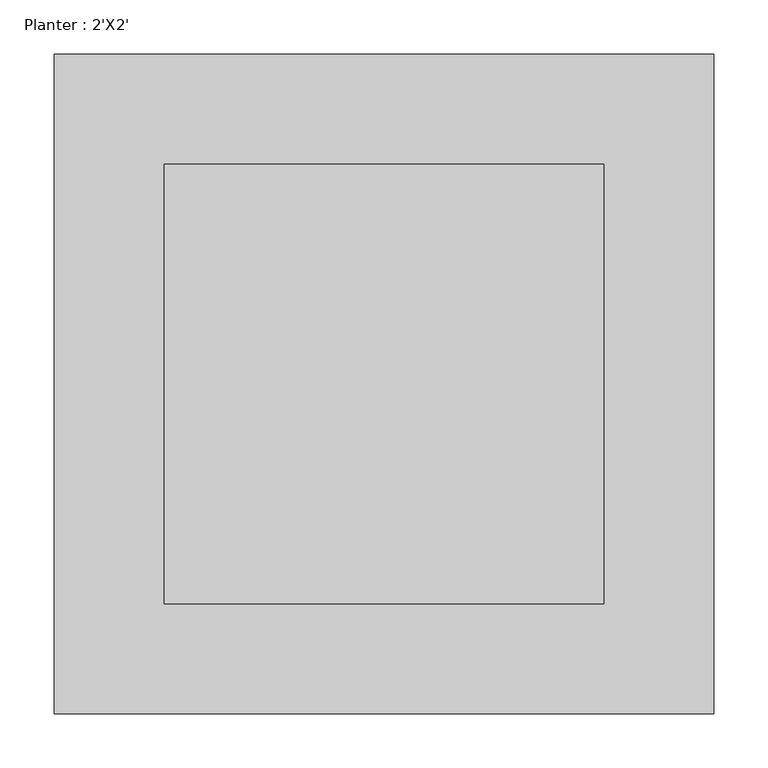
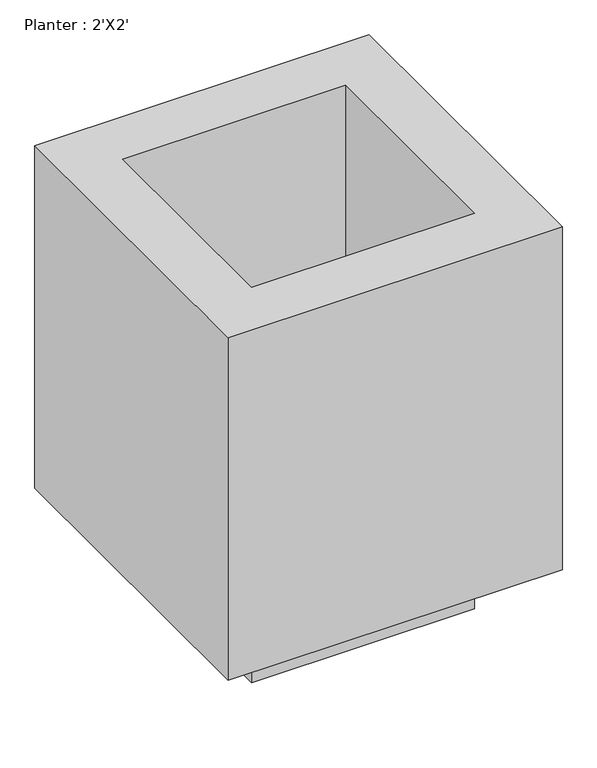
"""IFC4 building model written with IfcOpenShell, lengths in millimetres: geographic element geometry, Planter : 2'X2'."""

from ifc_helpers import new_model, si_unit, origin, origin_with_axes, place, context, project, spatial, polyline, outline, extrude, faceted_brep, source, transform, mapped, element, save


def planter_2_x2_5b049b04(model_context):
    return source(origin(), model_context, "Body", "SolidModel", [
        faceted_brep([(304.8, 304.8, 762.0), (-304.8, 304.8, 762.0), (-304.8, -304.8, 762.0), (304.8, -304.8, 762.0), (-203.2, 203.2, 762.0), (203.2, 203.2, 762.0), (203.2, -203.2, 762.0), (-203.2, -203.2, 762.0), (304.8, 304.8, 101.6), (304.8, -304.8, 101.6), (-304.8, -304.8, 101.6), (-304.8, 304.8, 101.6), (203.2, 203.2, 203.2), (-203.2, 203.2, 203.2), (-203.2, -203.2, 203.2), (203.2, -203.2, 203.2)], [[[0, 1, 2, 3], [4, 5, 6, 7]], [[8, 9, 10, 11]], [[1, 0, 8, 11]], [[2, 1, 11, 10]], [[3, 2, 10, 9]], [[0, 3, 9, 8]], [[12, 13, 14, 15]], [[13, 12, 5, 4]], [[14, 13, 4, 7]], [[15, 14, 7, 6]], [[12, 15, 6, 5]]]),
        extrude(outline(polyline([(203.2, 203.2), (203.2, -203.2), (-203.2, -203.2), (-203.2, 203.2), (203.2, 203.2)])), origin_with_axes(), (0.0, 0.0, 1.0), 101.6),
    ])


if __name__ == "__main__":
    model = new_model("IFC4")
    model_context = context("Model", 3, world=origin())
    ifc_project = project(units=[si_unit("LENGTHUNIT", "METRE", prefix="MILLI")], contexts=[model_context])
    site = spatial("IfcSite", under=ifc_project)
    building = spatial("IfcBuilding", under=site)
    placement = place(None, origin())
    planter_2_x2_shape = planter_2_x2_5b049b04(model_context)
    element("IfcGeographicElement", 1, ObjectType="Planter : 2'X2'", at=placement, inside=building, context=model_context, shape_type="MappedRepresentation", body=[
        mapped(planter_2_x2_shape, transform((0.0, 0.0, 0.0), x_axis=(1.0, 0.0, 0.0), y_axis=(0.0, 1.0, 0.0), z_axis=(0.0, 0.0, 1.0))),
    ])
    save(model, "model.ifc")

# Revit data of these elements
# Type "Planter : 2'X2'"
#   Depth = 2' - 0"
#   Height = 2' - 6"
#   Width = 2' - 0"
#   Material = Concrete, Precast
# Element 1 (IfcGeographicElement, "Planter : 2'X2'")
#   Materials on its faces: "Concrete, Precast"
# Materials
#   "Concrete, Precast": class "Concrete", colour RGB 198 187 187, transparency 0, Description = "Precast concrete", Cost = 0
